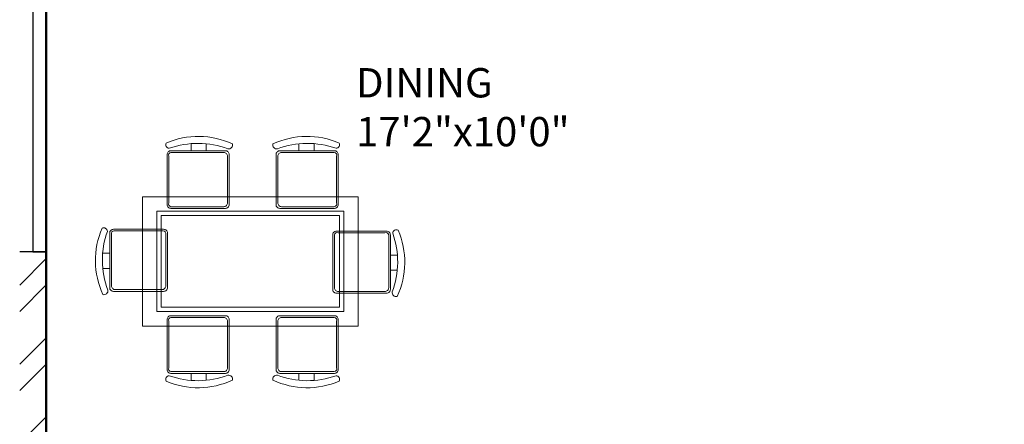
# Model space of a CAD drawing. Units: inches. Extents: x 1901 to 2863, y 888 to 2433.
# Tile 32 of 91: x 2439 to 2607, y 1405 to 1474. Entities that reach past the tile are written whole.
import ezdxf

# ---------------------------------------------------------------- set-up
doc = ezdxf.new("R2010")
doc.units = ezdxf.units.IN
for name, color, linetype, lineweight in [('A-AREA-IDEN', 7, 'Continuous', 18), ('A-FURN', 8, 'Continuous', 18), ('A-GLAZ', 3, 'Continuous', 25), ('A-WALL', 7, 'Continuous', 50), ('A-WALL-PATT', 8, 'Continuous', 13)]:
    doc.layers.add(name, color=color, linetype=linetype, lineweight=lineweight)
doc.styles.get("Standard").update_dxf_attribs({"font": 'arial.ttf'})

# ---------------------------------------------------------------- blocks, each defined once
blk = doc.blocks.new('WIN-60')
for p, q in [((0, 4.5), (0, 0)), ((60, 2.25), (60, 4.5)), ((60, 4.5), (60, 0)), ((0, 0), (0, 2.25)), ((0, 2.25), (60, 2.25))]:
    blk.add_line(p, q)

msp = doc.modelspace()

# ---------------------------------------------------------------- hatches: boundary and pattern name
at = {"layer": 'A-WALL-PATT'}
h = msp.add_hatch(dxfattribs=at)
h.set_pattern_fill('ANSI32', color=256)
h.paths.add_polyline_path([(2192.5, 2274.13), (2141.26, 2274.13), (2141.26, 2269.63), (2192.5, 2269.63)])
h.paths.add_polyline_path([(2259.93, 2274.13), (2216.5, 2274.13), (2216.5, 2269.63), (2255.43, 2269.63), (2255.43, 2214.63), (2250.81, 2214.63), (2250.81, 2210.13), (2259.93, 2210.13), (2259.93, 2215.13), (2271.76, 2215.13), (2271.76, 2217.38), (2271.76, 2219.63), (2259.93, 2219.63)])
h.paths.add_polyline_path([(2171.43, 2269.63), (2166.93, 2269.63), (2166.93, 2219.63), (2121.24, 2219.63), (2121.24, 2215.13), (2166.93, 2215.13), (2166.93, 2083.13), (2161.81, 2083.13), (2161.81, 2078.63), (2171.43, 2078.63), (2177, 2078.63), (2177, 2080.88), (2177, 2083.13), (2171.43, 2083.13), (2171.43, 2210.13), (2230.91, 2210.13), (2230.91, 2212.38), (2230.91, 2214.63), (2171.43, 2214.63)])
h.paths.add_polyline_path([(2117.26, 2274.13), (2089.43, 2274.13), (2089.43, 2219.63), (2081.14, 2219.63), (2081.14, 2215.13), (2089.43, 2215.13), (2098, 2215.13), (2098, 2217.38), (2098, 2219.63), (2093.93, 2219.63), (2093.93, 2269.63), (2117.26, 2269.63), (2117.26, 2271.88)])
h.paths.add_polyline_path([(2343.43, 2219.63), (2329.29, 2219.63), (2329.29, 2215.13), (2338.93, 2215.13), (2338.93, 2184.74), (2343.43, 2184.74)])
h.paths.add_polyline_path([(2338.93, 2083.13), (2329.29, 2083.13), (2208.97, 2083.13), (2208.97, 2078.63), (2338.93, 2078.63)])
h.paths.add_polyline_path([(2343.43, 2136.74), (2338.93, 2136.74), (2338.93, 1872.63), (2343.43, 1872.63)])
h.paths.add_polyline_path([(2343.43, 1863.63), (2397.68, 1863.63), (2397.68, 1821.63), (2384.14, 1821.63), (2384.14, 1812.63), (2418.33, 1812.63), (2418.33, 1817.13), (2418.33, 1821.63), (2406.68, 1821.63), (2406.68, 1863.63), (2459.5, 1863.63), (2459.5, 1821.63), (2447.14, 1821.63), (2447.14, 1812.63), (2459.5, 1812.63), (2468.5, 1812.63), (2468.5, 1872.63), (2394.43, 1872.63), (2334.43, 1872.63), (2334.43, 1812.63), (2343.43, 1812.63), (2353.25, 1812.63), (2353.25, 1821.63), (2343.43, 1821.63)])
h.paths.add_polyline_path([(2510.01, 1872.63), (2468.5, 1872.63), (2468.5, 1868.13), (2510.01, 1868.13)])
h.paths.add_polyline_path([(2514.01, 1817.13), (2468.5, 1817.13), (2468.5, 1812.63), (2482.11, 1812.63), (2482.11, 1800.61), (2486.61, 1800.61), (2486.61, 1812.63), (2514.01, 1812.63)])
h.paths.add_polyline_path([(2299.25, 1814.88), (2299.25, 1817.13), (2295.93, 1817.13), (2295.93, 1854.17), (2293.68, 1854.17), (2291.43, 1854.17), (2291.43, 1817.13), (2266.11, 1817.13), (2266.11, 1812.63), (2299.25, 1812.63)])
h.paths.add_polyline_path([(2218.11, 1817.13), (2206.46, 1817.13), (2171.43, 1817.13), (2171.43, 1949.13), (2190.1, 1949.13), (2190.1, 1953.63), (2163.47, 1953.63), (2163.47, 1949.13), (2166.93, 1949.13), (2166.93, 1817.13), (2114.3, 1817.13), (2114.3, 1812.63), (2218.11, 1812.63)])
h.paths.add_polyline_path([(2029.43, 1970.92), (2024.93, 1970.92), (2024.93, 1912.72), (2029.43, 1912.72)])
h.paths.add_polyline_path([(2132.3, 1953.63), (2113.93, 1953.63), (2113.93, 1975.89), (2111.68, 1975.89), (2109.43, 1975.89), (2109.43, 1953.63), (2029.43, 1953.63), (2029.43, 1949.13), (2132.3, 1949.13)])
h.paths.add_polyline_path([(2029.43, 1853.61), (2029.31, 1853.61), (2029.31, 1853.61), (2029.43, 1853.61), (2029.43, 1864.72), (2024.93, 1864.72), (2024.93, 1812.63), (2066.3, 1812.63), (2066.3, 1814.88), (2066.3, 1817.13), (2029.43, 1817.13)])
h.paths.add_polyline_path([(2122.93, 2010.09), (2120.68, 2010.09), (2118.43, 2010.09), (2118.43, 2006.13), (2029.43, 2006.13), (2029.43, 2001.63), (2109.43, 2001.63), (2109.43, 1998.04), (2113.93, 1998.04), (2113.93, 2001.63), (2122.93, 2001.63)])
h.paths.add_polyline_path([(2029.43, 2031.38), (2024.93, 2031.38), (2024.93, 1994.92), (2027.18, 1994.92), (2029.43, 1994.92)])
h.paths.add_polyline_path([(2029.43, 2136.74), (2024.93, 2136.74), (2024.93, 2067.38), (2027.18, 2067.38), (2029.43, 2067.38)])
h.paths.add_polyline_path([(2125.62, 2083.13), (2029.43, 2083.13), (2029.43, 2078.63), (2118.43, 2078.63), (2118.43, 2030.71), (2122.93, 2030.71), (2122.93, 2078.63), (2125.62, 2078.63)])
h.paths.add_polyline_path([(2029.43, 2215.13), (2040.47, 2215.13), (2040.47, 2217.38), (2040.47, 2219.63), (2024.93, 2219.63), (2024.93, 2184.74), (2029.43, 2184.74), (2029.43, 2187.78)])
h.paths.add_polyline_path([(2686.43, 2274.13), (2659.28, 2274.13), (2659.28, 2269.63), (2681.93, 2269.63), (2681.93, 2219.63), (2676.82, 2219.63), (2676.82, 2215.13), (2681.93, 2215.13), (2697.01, 2215.13), (2697.01, 2217.38), (2697.01, 2219.63), (2686.43, 2219.63)])
h.paths.add_polyline_path([(2609.93, 2269.63), (2635.28, 2269.63), (2635.28, 2274.13), (2571.43, 2274.13), (2571.43, 2269.63), (2605.43, 2269.63), (2605.43, 2214.63), (2549.1, 2214.63), (2549.1, 2210.13), (2605.43, 2210.13), (2605.43, 2083.13), (2601.01, 2083.13), (2601.01, 2080.88), (2601.01, 2078.63), (2609.93, 2078.63), (2616.16, 2078.63), (2616.16, 2080.88), (2616.16, 2083.13), (2609.93, 2083.13), (2609.93, 2215.13), (2651.46, 2215.13), (2651.46, 2217.38), (2651.46, 2219.63), (2609.93, 2219.63)])
h.paths.add_polyline_path([(2521.43, 2269.63), (2547.43, 2269.63), (2547.43, 2271.88), (2547.43, 2274.13), (2516.93, 2274.13), (2516.93, 2219.63), (2506.41, 2219.63), (2506.41, 2215.13), (2516.93, 2215.13), (2516.93, 2210.13), (2525.4, 2210.13), (2525.4, 2212.38), (2525.4, 2214.63), (2521.43, 2214.63)])
h.paths.add_polyline_path([(2456.01, 2219.63), (2439.43, 2219.63), (2439.43, 2187.89), (2443.93, 2187.89), (2443.93, 2215.13), (2456.01, 2215.13)])
h.paths.add_polyline_path([(2752.93, 2219.63), (2739.48, 2219.63), (2739.48, 2215.13), (2748.43, 2215.13), (2748.43, 2187.89), (2752.93, 2187.89)])
h.paths.add_polyline_path([(2752.93, 2139.89), (2748.43, 2139.89), (2748.43, 2083.13), (2648.42, 2083.13), (2648.42, 2078.63), (2654.93, 2078.63), (2654.93, 2039.44), (2659.43, 2039.44), (2659.43, 2078.63), (2748.43, 2078.63), (2748.43, 2063.43), (2752.93, 2063.43)])
h.paths.add_polyline_path([(2752.93, 2010.63), (2659.43, 2010.63), (2659.43, 2015.65), (2654.93, 2015.65), (2654.93, 2010.63), (2605.43, 2010.63), (2605.43, 1920.97), (2609.93, 1920.97), (2609.93, 2006.13), (2748.43, 2006.13), (2748.43, 1982.47), (2752.93, 1982.47)])
h.paths.add_polyline_path([(2752.93, 2027.43), (2748.43, 2027.43), (2748.43, 2010.63), (2752.93, 2010.63)])
h.paths.add_polyline_path([(2748.43, 1886.13), (2609.93, 1886.13), (2609.93, 1889.72), (2605.43, 1889.72), (2605.43, 1861.26), (2609.93, 1861.26), (2609.93, 1881.63), (2748.43, 1881.63)])
h.paths.add_polyline_path([(2456.86, 2228.83), (2498.4, 2228.83), (2498.4, 2247.49), (2456.86, 2247.49)], flags=9)
h.paths.add_polyline_path([(2038.6, 2237.42), (2080.17, 2237.42), (2080.17, 2256.08), (2038.6, 2256.08)], flags=9)
h.paths.add_polyline_path([(2292.01, 1062.39), (2539.93, 1062.39), (2539.93, 1099.49), (2292.01, 1099.49)], flags=9)
h.paths.add_polyline_path([(2424.91, 1832.25), (2448.51, 1832.25), (2448.51, 1846.68), (2424.91, 1846.68)], flags=25)
h.paths.add_polyline_path([(2359.08, 1832.25), (2382.68, 1832.25), (2382.68, 1846.68), (2359.08, 1846.68)], flags=25)
h.paths.add_polyline_path([(2352.9, 1684.8), (2367.54, 1684.8), (2367.54, 1697.17), (2352.9, 1697.17)], flags=9)
h.paths.add_polyline_path([(2079.29, 1755.83), (2169.02, 1755.83), (2169.02, 1774.37), (2079.29, 1774.37)], flags=9)
h.paths.add_polyline_path([(2404.09, 1373.86), (2404.09, 1463.59), (2385.54, 1463.59), (2385.54, 1373.86)], flags=9)
h.paths.add_polyline_path([(2268.09, 2236.37), (2309.64, 2236.37), (2309.64, 2255.03), (2268.09, 2255.03)], flags=9)
h.paths.add_polyline_path([(2575.96, 1700.95), (2665.7, 1700.95), (2665.7, 1719.5), (2575.96, 1719.5)], flags=9)
h.paths.add_polyline_path([(2302.96, 1878.47), (2329.52, 1878.47), (2329.52, 1888.78), (2302.96, 1888.78)], flags=9)
h.paths.add_polyline_path([(2097.42, 2240.58), (2126.57, 2240.58), (2126.57, 2259.23), (2097.42, 2259.23)], flags=9)
h.paths.add_polyline_path([(2208.72, 2246.12), (2237.88, 2246.12), (2237.88, 2264.78), (2208.72, 2264.78)], flags=9)
h.paths.add_polyline_path([(2038.15, 1925.96), (2076.99, 1925.96), (2076.99, 1944.62), (2038.15, 1944.62)], flags=9)
h.paths.add_polyline_path([(2239.14, 1926.67), (2288.46, 1926.67), (2288.46, 1945.33), (2239.14, 1945.33)], flags=9)
h.paths.add_polyline_path([(2175.43, 2007.33), (2212.36, 2007.33), (2212.36, 2025.99), (2175.43, 2025.99)], flags=9)
h.paths.add_polyline_path([(2225.03, 2091.79), (2263.87, 2091.79), (2263.87, 2110.45), (2225.03, 2110.45)], flags=9)
h.paths.add_polyline_path([(2035.4, 2098.48), (2074.24, 2098.48), (2074.24, 2117.14), (2035.4, 2117.14)], flags=9)
h.paths.add_polyline_path([(2050.1, 2029.21), (2083.26, 2029.21), (2083.26, 2047.87), (2050.1, 2047.87)], flags=9)
h.paths.add_polyline_path([(2069.68, 1956.72), (2098.83, 1956.72), (2098.83, 1975.38), (2069.68, 1975.38)], flags=25)
h.paths.add_polyline_path([(2328.62, 1753.34), (2361.66, 1753.34), (2361.66, 1771.99), (2328.62, 1771.99)], flags=9)
h.paths.add_polyline_path([(2395.16, 2060.89), (2395.16, 2140.65), (2378.68, 2140.65), (2378.68, 2060.89)], flags=9)
h.paths.add_polyline_path([(2463.73, 2059.02), (2492.89, 2059.02), (2492.89, 2077.68), (2463.73, 2077.68)], flags=9)
h.paths.add_polyline_path([(2458.03, 2181.54), (2496.87, 2181.54), (2496.87, 2200.19), (2458.03, 2200.19)], flags=9)
h.paths.add_polyline_path([(2527.58, 2243.07), (2556.73, 2243.07), (2556.73, 2261.73), (2527.58, 2261.73)], flags=9)
h.paths.add_polyline_path([(2694.46, 2232.77), (2736.03, 2232.77), (2736.03, 2251.42), (2694.46, 2251.42)], flags=9)
h.paths.add_polyline_path([(2637.82, 2249.22), (2666.98, 2249.22), (2666.98, 2267.88), (2637.82, 2267.88)], flags=9)
h.paths.add_polyline_path([(2623.69, 2183.54), (2662.53, 2183.54), (2662.53, 2202.2), (2623.69, 2202.2)], flags=9)
h.paths.add_polyline_path([(2691.97, 2021.5), (2725.12, 2021.5), (2725.12, 2040.16), (2691.97, 2040.16)], flags=9)
h.paths.add_polyline_path([(2621.04, 1975.91), (2662.34, 1975.91), (2662.34, 1994.57), (2621.04, 1994.57)], flags=25)
h.paths.add_polyline_path([(2479.03, 1927.62), (2519.84, 1927.62), (2519.84, 1946.28), (2479.03, 1946.28)], flags=9)
h.paths.add_polyline_path([(2670.94, 1849.08), (2716.01, 1849.08), (2716.01, 1867.73), (2670.94, 1867.73)], flags=9)
h.paths.add_polyline_path([(2523.61, 1782.96), (2550.17, 1782.96), (2550.17, 1793.26), (2523.61, 1793.26)], flags=9)
h.paths.add_polyline_path([(2450.84, 1207.33), (2492.39, 1207.33), (2492.39, 1225.99), (2450.84, 1225.99)], flags=9)
h.paths.add_polyline_path([(2527.75, 1203.84), (2556.91, 1203.84), (2556.91, 1222.5), (2527.75, 1222.5)], flags=9)
h.paths.add_polyline_path([(2639.11, 1207.2), (2668.27, 1207.2), (2668.27, 1225.86), (2639.11, 1225.86)], flags=9)
h.paths.add_polyline_path([(2692.59, 1218.97), (2734.17, 1218.97), (2734.17, 1237.62), (2692.59, 1237.62)], flags=9)
h.paths.add_polyline_path([(2669.27, 1366.33), (2708.11, 1366.33), (2708.11, 1384.99), (2669.27, 1384.99)], flags=9)
h.paths.add_polyline_path([(2463.31, 1358.03), (2502.15, 1358.03), (2502.15, 1376.69), (2463.31, 1376.69)], flags=9)
h.paths.add_polyline_path([(2494.72, 1449.96), (2531.65, 1449.96), (2531.65, 1468.62), (2494.72, 1468.62)], flags=9)
h.paths.add_polyline_path([(2675.57, 1422.16), (2708.72, 1422.16), (2708.72, 1440.81), (2675.57, 1440.81)], flags=9)
h.paths.add_polyline_path([(2685.63, 1493.89), (2714.79, 1493.89), (2714.79, 1512.55), (2685.63, 1512.55)], flags=9)
h.paths.add_polyline_path([(2686.8, 1529.91), (2725.65, 1529.91), (2725.65, 1548.57), (2686.8, 1548.57)], flags=9)
h.paths.add_polyline_path([(2503.65, 1537.99), (2552.97, 1537.99), (2552.97, 1556.65), (2503.65, 1556.65)], flags=9)
h.paths.add_polyline_path([(2291.71, 1643.5), (2318.28, 1643.5), (2318.28, 1653.81), (2291.71, 1653.81)], flags=9)
h.paths.add_polyline_path([(2450.63, 1610.52), (2477.19, 1610.52), (2477.19, 1620.82), (2450.63, 1620.82)], flags=9)
h.paths.add_polyline_path([(2359.99, 1551.81), (2422.25, 1551.81), (2422.25, 1562.12), (2359.99, 1562.12)], flags=9)
h.paths.add_polyline_path([(2280.11, 1249.01), (2321.65, 1249.01), (2321.65, 1267.66), (2280.11, 1267.66)], flags=9)
h.paths.add_polyline_path([(2164.06, 1274.23), (2193.22, 1274.23), (2193.22, 1292.89), (2164.06, 1292.89)], flags=9)
h.paths.add_polyline_path([(2118.21, 1277.69), (2151.25, 1277.69), (2151.25, 1296.35), (2118.21, 1296.35)], flags=9)
h.paths.add_polyline_path([(2031.95, 1268.53), (2073.52, 1268.53), (2073.52, 1287.19), (2031.95, 1287.19)], flags=9)
h.paths.add_polyline_path([(2050.2, 1409.08), (2089.04, 1409.08), (2089.04, 1427.74), (2050.2, 1427.74)], flags=9)
h.paths.add_polyline_path([(2243.74, 1421.03), (2282.58, 1421.03), (2282.58, 1439.69), (2243.74, 1439.69)], flags=9)
h.paths.add_polyline_path([(2190.75, 1509.77), (2231.56, 1509.77), (2231.56, 1528.43), (2190.75, 1528.43)], flags=9)
h.paths.add_polyline_path([(2058.39, 1475.42), (2091.55, 1475.42), (2091.55, 1494.07), (2058.39, 1494.07)], flags=9)
h.paths.add_polyline_path([(2062.45, 1553.09), (2091.6, 1553.09), (2091.6, 1571.75), (2062.45, 1571.75)], flags=9)
h.paths.add_polyline_path([(2219.52, 1590.37), (2266.15, 1590.37), (2266.15, 1609.02), (2219.52, 1609.02)], flags=9)
h.paths.add_polyline_path([(2041.07, 1584.19), (2079.91, 1584.19), (2079.91, 1602.85), (2041.07, 1602.85)], flags=9)
h = msp.add_hatch(dxfattribs=at)
h.set_pattern_fill('ANSI32', color=256)
h.paths.add_polyline_path([(2443.93, 2139.89), (2439.43, 2139.89), (2439.43, 2069.35), (2441.68, 2069.35), (2443.93, 2069.35), (2443.93, 2078.63), (2521.93, 2078.63), (2521.93, 2075.07), (2524.18, 2075.07), (2526.43, 2075.07), (2526.43, 2078.63), (2571.75, 2078.63), (2571.75, 2080.88), (2571.75, 2083.13), (2443.93, 2083.13)])
h.paths.add_polyline_path([(2526.43, 2054.63), (2524.18, 2054.63), (2521.93, 2054.63), (2521.93, 2030.63), (2443.93, 2030.63), (2443.93, 2045.35), (2439.43, 2045.35), (2439.43, 1983.87), (2443.93, 1983.87), (2443.93, 2026.13), (2521.93, 2026.13), (2526.43, 2026.13)])
h.paths.add_polyline_path([(2443.93, 1923.87), (2439.43, 1923.87), (2439.43, 1872.63), (2443.93, 1872.63)])
h.paths.add_polyline_path([(2636.23, 1766.13), (2609.93, 1766.13), (2609.93, 1779.79), (2605.43, 1779.79), (2605.43, 1766.13), (2486.61, 1766.13), (2486.61, 1770.67), (2482.11, 1770.67), (2482.11, 1766.13), (2482.11, 1761.63), (2636.23, 1761.63), (2636.23, 1763.88)])
h.paths.add_polyline_path([(2519.54, 1663.38), (2519.54, 1665.63), (2494.93, 1665.63), (2481.83, 1665.63), (2481.83, 1663.38), (2481.83, 1661.13), (2490.43, 1661.13), (2490.43, 1640.16), (2494.93, 1640.16), (2494.93, 1661.13), (2519.54, 1661.13)])
h.paths.add_polyline_path([(2443.93, 1712.13), (2443.93, 1716.63), (2414.46, 1716.63), (2414.46, 1712.13), (2439.43, 1712.13), (2439.43, 1545.51), (2443.93, 1545.51), (2443.93, 1661.13), (2448.47, 1661.13), (2448.47, 1665.63), (2443.93, 1665.63)])
h.paths.add_polyline_path([(2343.43, 1712.13), (2365.52, 1712.13), (2365.52, 1714.38), (2365.52, 1716.63), (2333.87, 1716.63), (2333.87, 1714.38), (2333.87, 1712.13), (2338.93, 1712.13), (2338.93, 1575.63), (2338.93, 1545.51), (2343.43, 1545.51), (2343.43, 1547.51), (2343.43, 1580.13)])
h.paths.add_polyline_path([(2752.93, 1665.63), (2579.54, 1665.63), (2579.54, 1661.13), (2615.93, 1661.13), (2615.93, 1529.13), (2598.93, 1529.13), (2598.93, 1524.63), (2623.13, 1524.63), (2623.13, 1526.88), (2623.13, 1529.13), (2620.43, 1529.13), (2620.43, 1661.13), (2748.43, 1661.13), (2748.43, 1633.5), (2752.93, 1633.5)])
h.paths.add_polyline_path([(2752.93, 1419.93), (2748.43, 1419.93), (2748.43, 1400.13), (2659.43, 1400.13), (2659.43, 1444.33), (2657.18, 1444.33), (2654.93, 1444.33), (2654.93, 1400.13), (2643.65, 1400.13), (2643.65, 1395.63), (2748.43, 1395.63), (2748.43, 1364.04), (2752.93, 1364.04)])
h.paths.add_polyline_path([(2752.93, 1492.88), (2748.43, 1492.88), (2748.43, 1476.63), (2667.43, 1476.63), (2667.43, 1479.71), (2665.18, 1479.71), (2662.93, 1479.71), (2662.93, 1476.63), (2654.93, 1476.63), (2654.93, 1469.54), (2659.43, 1469.54), (2659.43, 1472.13), (2748.43, 1472.13), (2748.43, 1455.93), (2752.93, 1455.93)])
h.paths.add_polyline_path([(2752.93, 1304.04), (2748.43, 1304.04), (2748.43, 1263.63), (2738.66, 1263.63), (2738.66, 1259.13), (2752.93, 1259.13)])
h.paths.add_polyline_path([(2685.93, 1259.13), (2695.49, 1259.13), (2695.49, 1261.38), (2695.49, 1263.63), (2677.84, 1263.63), (2677.84, 1261.38), (2677.84, 1259.13), (2681.43, 1259.13), (2681.43, 1203.63), (2653.28, 1203.63), (2653.28, 1199.13), (2685.93, 1199.13), (2685.93, 1203.63)])
h.paths.add_polyline_path([(2609.43, 1395.63), (2611.85, 1395.63), (2611.85, 1400.13), (2598.89, 1400.13), (2598.89, 1397.88), (2598.89, 1395.63), (2604.93, 1395.63), (2604.93, 1268.13), (2554.73, 1268.13), (2554.73, 1265.88), (2554.73, 1263.63), (2604.93, 1263.63), (2604.93, 1203.63), (2571.31, 1203.63), (2571.31, 1199.13), (2604.93, 1199.13), (2629.28, 1199.13), (2629.28, 1201.38), (2629.28, 1203.63), (2609.43, 1203.63), (2609.43, 1258.63), (2609.43, 1259.13), (2654.8, 1259.13), (2654.8, 1263.63), (2609.43, 1263.63)])
h.paths.add_polyline_path([(2443.93, 1304.04), (2439.43, 1304.04), (2439.43, 1259.13), (2443.93, 1259.13), (2456.16, 1259.13), (2456.16, 1261.38), (2456.16, 1263.63), (2443.93, 1263.63)])
h.paths.add_polyline_path([(2525.43, 1263.63), (2531.78, 1263.63), (2531.78, 1268.13), (2520.93, 1268.13), (2520.93, 1263.63), (2511.41, 1263.63), (2511.41, 1259.13), (2520.93, 1259.13), (2520.93, 1199.13), (2547.31, 1199.13), (2547.31, 1201.38), (2547.31, 1203.63), (2525.43, 1203.63)])
h.paths.add_polyline_path([(2443.93, 1434.84), (2439.43, 1434.84), (2439.43, 1364.04), (2441.68, 1364.04), (2443.93, 1364.04)])
h.paths.add_polyline_path([(2567.13, 1400.13), (2443.93, 1400.13), (2443.93, 1395.63), (2567.13, 1395.63)])
h.paths.add_polyline_path([(2443.93, 1545.51), (2439.43, 1545.51), (2439.43, 1494.84), (2443.93, 1494.84)])
h.paths.add_polyline_path([(2494.93, 1553.35), (2492.68, 1553.35), (2490.43, 1553.35), (2490.43, 1524.63), (2494.93, 1524.63), (2525.94, 1524.63), (2525.94, 1526.88), (2525.94, 1529.13), (2494.93, 1529.13)])
h.paths.add_polyline_path([(2752.93, 1573.5), (2748.43, 1573.5), (2748.43, 1529.13), (2657.76, 1529.13), (2657.76, 1524.63), (2662.93, 1524.63), (2662.93, 1498.63), (2667.43, 1498.63), (2667.43, 1524.63), (2748.43, 1524.63), (2748.43, 1516.88), (2752.93, 1516.88)])
h.paths.add_polyline_path([(2038.6, 2237.42), (2080.17, 2237.42), (2080.17, 2256.08), (2038.6, 2256.08)], flags=9)
h.paths.add_polyline_path([(2292.01, 1062.39), (2539.93, 1062.39), (2539.93, 1099.49), (2292.01, 1099.49)], flags=9)
h.paths.add_polyline_path([(2424.91, 1832.25), (2448.51, 1832.25), (2448.51, 1846.68), (2424.91, 1846.68)], flags=9)
h.paths.add_polyline_path([(2359.08, 1832.25), (2382.68, 1832.25), (2382.68, 1846.68), (2359.08, 1846.68)], flags=9)
h.paths.add_polyline_path([(2352.9, 1684.8), (2367.54, 1684.8), (2367.54, 1697.17), (2352.9, 1697.17)], flags=9)
h.paths.add_polyline_path([(2079.29, 1755.83), (2169.02, 1755.83), (2169.02, 1774.37), (2079.29, 1774.37)], flags=9)
h.paths.add_polyline_path([(2404.09, 1373.86), (2404.09, 1463.59), (2385.54, 1463.59), (2385.54, 1373.86)], flags=9)
h.paths.add_polyline_path([(2268.09, 2236.37), (2309.64, 2236.37), (2309.64, 2255.03), (2268.09, 2255.03)], flags=9)
h.paths.add_polyline_path([(2575.96, 1700.95), (2665.7, 1700.95), (2665.7, 1719.5), (2575.96, 1719.5)], flags=9)
h.paths.add_polyline_path([(2302.96, 1878.47), (2329.52, 1878.47), (2329.52, 1888.78), (2302.96, 1888.78)], flags=9)
h.paths.add_polyline_path([(2097.42, 2240.58), (2126.57, 2240.58), (2126.57, 2259.23), (2097.42, 2259.23)], flags=9)
h.paths.add_polyline_path([(2208.72, 2246.12), (2237.88, 2246.12), (2237.88, 2264.78), (2208.72, 2264.78)], flags=9)
h.paths.add_polyline_path([(2038.15, 1925.96), (2076.99, 1925.96), (2076.99, 1944.62), (2038.15, 1944.62)], flags=9)
h.paths.add_polyline_path([(2239.14, 1926.67), (2288.46, 1926.67), (2288.46, 1945.33), (2239.14, 1945.33)], flags=9)
h.paths.add_polyline_path([(2175.43, 2007.33), (2212.36, 2007.33), (2212.36, 2025.99), (2175.43, 2025.99)], flags=9)
h.paths.add_polyline_path([(2225.03, 2091.79), (2263.87, 2091.79), (2263.87, 2110.45), (2225.03, 2110.45)], flags=9)
h.paths.add_polyline_path([(2035.4, 2098.48), (2074.24, 2098.48), (2074.24, 2117.14), (2035.4, 2117.14)], flags=9)
h.paths.add_polyline_path([(2050.1, 2029.21), (2083.26, 2029.21), (2083.26, 2047.87), (2050.1, 2047.87)], flags=9)
h.paths.add_polyline_path([(2069.68, 1956.72), (2098.83, 1956.72), (2098.83, 1975.38), (2069.68, 1975.38)], flags=9)
h.paths.add_polyline_path([(2328.62, 1753.34), (2361.66, 1753.34), (2361.66, 1771.99), (2328.62, 1771.99)], flags=9)
h.paths.add_polyline_path([(2395.16, 2060.89), (2395.16, 2140.65), (2378.68, 2140.65), (2378.68, 2060.89)], flags=9)
h.paths.add_polyline_path([(2463.73, 2059.02), (2492.89, 2059.02), (2492.89, 2077.68), (2463.73, 2077.68)], flags=9)
h.paths.add_polyline_path([(2458.03, 2181.54), (2496.87, 2181.54), (2496.87, 2200.19), (2458.03, 2200.19)], flags=9)
h.paths.add_polyline_path([(2456.86, 2228.83), (2498.4, 2228.83), (2498.4, 2247.49), (2456.86, 2247.49)], flags=9)
h.paths.add_polyline_path([(2527.58, 2243.07), (2556.73, 2243.07), (2556.73, 2261.73), (2527.58, 2261.73)], flags=9)
h.paths.add_polyline_path([(2694.46, 2232.77), (2736.03, 2232.77), (2736.03, 2251.42), (2694.46, 2251.42)], flags=9)
h.paths.add_polyline_path([(2637.82, 2249.22), (2666.98, 2249.22), (2666.98, 2267.88), (2637.82, 2267.88)], flags=9)
h.paths.add_polyline_path([(2623.69, 2183.54), (2662.53, 2183.54), (2662.53, 2202.2), (2623.69, 2202.2)], flags=9)
h.paths.add_polyline_path([(2691.97, 2021.5), (2725.12, 2021.5), (2725.12, 2040.16), (2691.97, 2040.16)], flags=9)
h.paths.add_polyline_path([(2621.04, 1975.91), (2662.34, 1975.91), (2662.34, 1994.57), (2621.04, 1994.57)], flags=9)
h.paths.add_polyline_path([(2479.03, 1927.62), (2519.84, 1927.62), (2519.84, 1946.28), (2479.03, 1946.28)], flags=9)
h.paths.add_polyline_path([(2670.94, 1849.08), (2716.01, 1849.08), (2716.01, 1867.73), (2670.94, 1867.73)], flags=9)
h.paths.add_polyline_path([(2523.61, 1782.96), (2550.17, 1782.96), (2550.17, 1793.26), (2523.61, 1793.26)], flags=9)
h.paths.add_polyline_path([(2450.84, 1207.33), (2492.39, 1207.33), (2492.39, 1225.99), (2450.84, 1225.99)], flags=9)
h.paths.add_polyline_path([(2527.75, 1203.84), (2556.91, 1203.84), (2556.91, 1222.5), (2527.75, 1222.5)], flags=9)
h.paths.add_polyline_path([(2639.11, 1207.2), (2668.27, 1207.2), (2668.27, 1225.86), (2639.11, 1225.86)], flags=9)
h.paths.add_polyline_path([(2692.59, 1218.97), (2734.17, 1218.97), (2734.17, 1237.62), (2692.59, 1237.62)], flags=9)
h.paths.add_polyline_path([(2669.27, 1366.33), (2708.11, 1366.33), (2708.11, 1384.99), (2669.27, 1384.99)], flags=25)
h.paths.add_polyline_path([(2463.31, 1358.03), (2502.15, 1358.03), (2502.15, 1376.69), (2463.31, 1376.69)], flags=9)
h.paths.add_polyline_path([(2494.72, 1449.96), (2531.65, 1449.96), (2531.65, 1468.62), (2494.72, 1468.62)], flags=9)
h.paths.add_polyline_path([(2675.57, 1422.16), (2708.72, 1422.16), (2708.72, 1440.81), (2675.57, 1440.81)], flags=25)
h.paths.add_polyline_path([(2685.63, 1493.89), (2714.79, 1493.89), (2714.79, 1512.55), (2685.63, 1512.55)], flags=9)
h.paths.add_polyline_path([(2686.8, 1529.91), (2725.65, 1529.91), (2725.65, 1548.57), (2686.8, 1548.57)], flags=25)
h.paths.add_polyline_path([(2503.65, 1537.99), (2552.97, 1537.99), (2552.97, 1556.65), (2503.65, 1556.65)], flags=9)
h.paths.add_polyline_path([(2291.71, 1643.5), (2318.28, 1643.5), (2318.28, 1653.81), (2291.71, 1653.81)], flags=9)
h.paths.add_polyline_path([(2450.63, 1610.52), (2477.19, 1610.52), (2477.19, 1620.82), (2450.63, 1620.82)], flags=9)
h.paths.add_polyline_path([(2359.99, 1551.81), (2422.25, 1551.81), (2422.25, 1562.12), (2359.99, 1562.12)], flags=9)
h.paths.add_polyline_path([(2280.11, 1249.01), (2321.65, 1249.01), (2321.65, 1267.66), (2280.11, 1267.66)], flags=9)
h.paths.add_polyline_path([(2164.06, 1274.23), (2193.22, 1274.23), (2193.22, 1292.89), (2164.06, 1292.89)], flags=9)
h.paths.add_polyline_path([(2118.21, 1277.69), (2151.25, 1277.69), (2151.25, 1296.35), (2118.21, 1296.35)], flags=9)
h.paths.add_polyline_path([(2031.95, 1268.53), (2073.52, 1268.53), (2073.52, 1287.19), (2031.95, 1287.19)], flags=9)
h.paths.add_polyline_path([(2050.2, 1409.08), (2089.04, 1409.08), (2089.04, 1427.74), (2050.2, 1427.74)], flags=9)
h.paths.add_polyline_path([(2243.74, 1421.03), (2282.58, 1421.03), (2282.58, 1439.69), (2243.74, 1439.69)], flags=9)
h.paths.add_polyline_path([(2190.75, 1509.77), (2231.56, 1509.77), (2231.56, 1528.43), (2190.75, 1528.43)], flags=9)
h.paths.add_polyline_path([(2058.39, 1475.42), (2091.55, 1475.42), (2091.55, 1494.07), (2058.39, 1494.07)], flags=9)
h.paths.add_polyline_path([(2062.45, 1553.09), (2091.6, 1553.09), (2091.6, 1571.75), (2062.45, 1571.75)], flags=9)
h.paths.add_polyline_path([(2219.52, 1590.37), (2266.15, 1590.37), (2266.15, 1609.02), (2219.52, 1609.02)], flags=9)
h.paths.add_polyline_path([(2041.07, 1584.19), (2079.91, 1584.19), (2079.91, 1602.85), (2041.07, 1602.85)], flags=9)

# ---------------------------------------------------------------- linework, layer by layer
at = {"layer": 'A-FURN'}
for points in [[(2464.9, 1452.46, -0.175809), (2474.9, 1452.38, 0.578392), (2475.66, 1453.21, 0.214524), (2464.37, 1453.36, 0.552014), (2464.9, 1452.46, -0.065079)], [(2464.9, 1452.46, -0.175809), (2474.9, 1452.38, 0.578392), (2475.66, 1453.21, 0.214524), (2464.37, 1453.36, 0.552014), (2464.9, 1452.46, -0.065079)], [(2483.33, 1452.38, -0.578392), (2482.57, 1453.21, -0.214524), (2493.86, 1453.36, -0.552014), (2493.33, 1452.46, 0.175809), (2483.33, 1452.38)], [(2483.33, 1452.38, -0.578392), (2482.57, 1453.21, -0.214524), (2493.86, 1453.36, -0.552014), (2493.33, 1452.46, 0.175809), (2483.33, 1452.38)], [(2471.22, 1452.05), (2471.22, 1453.23, -0.064759)], [(2471.22, 1452.05), (2471.22, 1453.23, -0.064759)], [(2487.01, 1452.05), (2487.01, 1453.23, 0.064759)], [(2487.01, 1452.05), (2487.01, 1453.23, 0.064759)], [(2474.48, 1452.05), (2465.19, 1452.05, 0.414214), (2464.54, 1451.4), (2464.54, 1442.87, 0.414214), (2465.19, 1442.22), (2474.48, 1442.22, 0.414214), (2475.13, 1442.87), (2475.13, 1451.4, 0.414214), (2474.48, 1452.05)], [(2474.48, 1452.05), (2465.19, 1452.05, 0.414214), (2464.54, 1451.4), (2464.54, 1442.87, 0.414214), (2465.19, 1442.22), (2474.48, 1442.22, 0.414214), (2475.13, 1442.87), (2475.13, 1451.4, 0.414214), (2474.48, 1452.05)], [(2493.04, 1452.05, -0.414214), (2493.69, 1451.4), (2493.69, 1442.87, -0.414214), (2493.04, 1442.22), (2483.75, 1442.22, -0.414214), (2483.1, 1442.87), (2483.1, 1451.4, -0.414214), (2483.75, 1452.05), (2493.04, 1452.05)], [(2493.04, 1452.05, -0.414214), (2493.69, 1451.4), (2493.69, 1442.87, -0.414214), (2493.04, 1442.22), (2483.75, 1442.22, -0.414214), (2483.1, 1442.87), (2483.1, 1451.4, -0.414214), (2483.75, 1452.05), (2493.04, 1452.05)], [(2454.43, 1428.3, -0.578392), (2453.6, 1427.54, -0.214524), (2453.45, 1438.83, -0.552014), (2454.36, 1438.3, 0.175809), (2454.43, 1428.3)], [(2454.43, 1428.3, -0.578392), (2453.6, 1427.54, -0.214524), (2453.45, 1438.83, -0.552014), (2454.36, 1438.3, 0.175809), (2454.43, 1428.3)], [(2454.76, 1438.01, -0.414214), (2455.41, 1438.66), (2463.95, 1438.66, -0.414214), (2464.6, 1438.01), (2464.6, 1428.72, -0.414214), (2463.95, 1428.07), (2455.41, 1428.07, -0.414214), (2454.76, 1428.72), (2454.76, 1438.01)], [(2454.76, 1438.01, -0.414214), (2455.41, 1438.66), (2463.95, 1438.66, -0.414214), (2464.6, 1438.01), (2464.6, 1428.72, -0.414214), (2463.95, 1428.07), (2455.41, 1428.07, -0.414214), (2454.76, 1428.72), (2454.76, 1438.01)], [(2502.58, 1437.69, 0.414214), (2501.93, 1438.34), (2493.39, 1438.34, 0.414214), (2492.75, 1437.69), (2492.75, 1428.41, 0.414214), (2493.39, 1427.76), (2501.93, 1427.76, 0.414214), (2502.58, 1428.41), (2502.58, 1437.69)], [(2502.58, 1437.69, 0.414214), (2501.93, 1438.34), (2493.39, 1438.34, 0.414214), (2492.75, 1437.69), (2492.75, 1428.4, 0.414214), (2493.39, 1427.75), (2501.93, 1427.75, 0.414214), (2502.58, 1428.4), (2502.58, 1437.69)], [(2502.99, 1437.98, -0.175809), (2502.91, 1427.98, 0.578392), (2503.74, 1427.22, 0.214524), (2503.89, 1438.51, 0.552014), (2502.99, 1437.98, -0.065079)], [(2502.99, 1437.98, -0.175809), (2502.91, 1427.98, 0.578392), (2503.74, 1427.22, 0.214524), (2503.89, 1438.51, 0.552014), (2502.99, 1437.98, -0.065079)], [(2454.76, 1431.99), (2453.59, 1431.99, 0.064759)], [(2454.76, 1431.98), (2453.59, 1431.98, 0.064759)], [(2502.58, 1431.67), (2503.76, 1431.67, -0.064759)], [(2502.58, 1431.67), (2503.76, 1431.67, -0.064759)], [(2474.48, 1414.1), (2465.19, 1414.1, -0.414214), (2464.54, 1414.75), (2464.54, 1423.28, -0.414214), (2465.19, 1423.93), (2474.48, 1423.93, -0.414214), (2475.13, 1423.28), (2475.13, 1414.75, -0.414214), (2474.48, 1414.1)], [(2474.48, 1414.1), (2465.19, 1414.1, -0.414214), (2464.54, 1414.74), (2464.54, 1423.28, -0.414214), (2465.19, 1423.93), (2474.48, 1423.93, -0.414214), (2475.13, 1423.28), (2475.13, 1414.74, -0.414214), (2474.48, 1414.1)], [(2493.04, 1414.1, 0.414214), (2493.69, 1414.75), (2493.69, 1423.28, 0.414214), (2493.04, 1423.93), (2483.75, 1423.93, 0.414214), (2483.1, 1423.28), (2483.1, 1414.75, 0.414214), (2483.75, 1414.1), (2493.04, 1414.1)], [(2493.04, 1414.1, 0.414214), (2493.69, 1414.74), (2493.69, 1423.28, 0.414214), (2493.04, 1423.93), (2483.75, 1423.93, 0.414214), (2483.1, 1423.28), (2483.1, 1414.74, 0.414214), (2483.75, 1414.1), (2493.04, 1414.1)], [(2474.9, 1413.77, -0.578392), (2475.66, 1412.94, -0.214524), (2464.37, 1412.78, -0.552014), (2464.9, 1413.69, 0.175809), (2474.9, 1413.77)], [(2474.9, 1413.77, -0.578392), (2475.66, 1412.94, -0.214524), (2464.37, 1412.78, -0.552014), (2464.9, 1413.69, 0.175809), (2474.9, 1413.77)], [(2471.22, 1414.1), (2471.22, 1412.92, 0.064759)], [(2471.22, 1414.1), (2471.22, 1412.92, 0.064759)], [(2493.33, 1413.69, -0.175809), (2483.33, 1413.77, 0.578392), (2482.57, 1412.94, 0.214524), (2493.86, 1412.78, 0.552014), (2493.33, 1413.69, -0.065079)], [(2493.33, 1413.69, -0.175809), (2483.33, 1413.77, 0.578392), (2482.57, 1412.94, 0.214524), (2493.86, 1412.78, 0.552014), (2493.33, 1413.69, -0.065079)], [(2487.01, 1414.1), (2487.01, 1412.92, -0.064759)], [(2487.01, 1414.1), (2487.01, 1412.92, -0.064759)]]:
    msp.add_lwpolyline(points, format="xyb", dxfattribs=at)
for points in [[(2468.62, 1453.25), (2468.62, 1452.05)], [(2468.62, 1453.25), (2468.62, 1452.05)], [(2489.61, 1453.25), (2489.61, 1452.05)], [(2489.61, 1453.25), (2489.61, 1452.05)], [(2453.56, 1434.58), (2454.76, 1434.58)], [(2453.56, 1434.58), (2454.76, 1434.58)], [(2503.78, 1434.27), (2502.58, 1434.27)], [(2503.78, 1434.27), (2502.58, 1434.27)], [(2468.62, 1412.9), (2468.62, 1414.1)], [(2468.62, 1412.9), (2468.62, 1414.1)], [(2489.61, 1412.9), (2489.61, 1414.1)], [(2489.61, 1412.9), (2489.61, 1414.1)]]:
    msp.add_lwpolyline(points, dxfattribs=at)
for points in [[(2465.2, 1451.76), (2474.19, 1451.76, -0.414214), (2474.84, 1451.11), (2474.84, 1443.16, -0.414214), (2474.19, 1442.51), (2465.2, 1442.51, -0.512069), (2464.84, 1443.16), (2464.84, 1451.11, -0.512069)], [(2465.2, 1451.76), (2474.19, 1451.76, -0.414214), (2474.84, 1451.11), (2474.84, 1443.16, -0.414214), (2474.19, 1442.51), (2465.2, 1442.51, -0.512069), (2464.84, 1443.16), (2464.84, 1451.11, -0.512069)], [(2493.03, 1451.76), (2484.04, 1451.76, 0.414214), (2483.39, 1451.11), (2483.39, 1443.16, 0.414214), (2484.04, 1442.51), (2493.03, 1442.51, 0.512069), (2493.39, 1443.16), (2493.39, 1451.11, 0.512069)], [(2493.03, 1451.76), (2484.04, 1451.76, 0.414214), (2483.39, 1451.11), (2483.39, 1443.16, 0.414214), (2484.04, 1442.51), (2493.03, 1442.51, 0.512069), (2493.39, 1443.16), (2493.39, 1451.11, 0.512069)], [(2455.05, 1438.01), (2455.05, 1429.02, 0.414214), (2455.7, 1428.37), (2463.66, 1428.37, 0.414214), (2464.31, 1429.02), (2464.31, 1438.01, 0.512069), (2463.66, 1438.37), (2455.7, 1438.37, 0.512069)], [(2455.05, 1438.01), (2455.05, 1429.02, 0.414214), (2455.7, 1428.37), (2463.66, 1428.37, 0.414214), (2464.31, 1429.02), (2464.31, 1438.01, 0.512069), (2463.66, 1438.37), (2455.7, 1438.37, 0.512069)], [(2502.29, 1437.69), (2502.29, 1428.7, -0.414214), (2501.64, 1428.05), (2493.69, 1428.05, -0.414214), (2493.04, 1428.7), (2493.04, 1437.69, -0.512069), (2493.69, 1438.05), (2501.64, 1438.05, -0.512069)], [(2502.29, 1437.69), (2502.29, 1428.7, -0.414214), (2501.64, 1428.05), (2493.69, 1428.05, -0.414214), (2493.04, 1428.7), (2493.04, 1437.69, -0.512069), (2493.69, 1438.05), (2501.64, 1438.05, -0.512069)], [(2465.2, 1414.39), (2474.19, 1414.39, 0.414214), (2474.84, 1415.04), (2474.84, 1422.99, 0.414214), (2474.19, 1423.64), (2465.2, 1423.64, 0.512069), (2464.84, 1422.99), (2464.84, 1415.04, 0.512069)], [(2465.2, 1414.39), (2474.19, 1414.39, 0.414214), (2474.84, 1415.04), (2474.84, 1422.99, 0.414214), (2474.19, 1423.64), (2465.2, 1423.64, 0.512069), (2464.84, 1422.99), (2464.84, 1415.04, 0.512069)], [(2493.03, 1414.39), (2484.04, 1414.39, -0.414214), (2483.39, 1415.04), (2483.39, 1422.99, -0.414214), (2484.04, 1423.64), (2493.03, 1423.64, -0.512069), (2493.39, 1422.99), (2493.39, 1415.04, -0.512069)], [(2493.03, 1414.39), (2484.04, 1414.39, -0.414214), (2483.39, 1415.04), (2483.39, 1422.99, -0.414214), (2484.04, 1423.64), (2493.03, 1423.64, -0.512069), (2493.39, 1422.99), (2493.39, 1415.04, -0.512069)]]:
    msp.add_lwpolyline(points, format="xyb", close=True, dxfattribs=at)
for points in [[(2460.36, 1444.21), (2497.08, 1444.21), (2497.08, 1422.17), (2460.36, 1422.17)], [(2460.36, 1444.21), (2497.08, 1444.21), (2497.08, 1422.17), (2460.36, 1422.17)], [(2462.81, 1441.76), (2494.64, 1441.76), (2494.64, 1424.62), (2462.81, 1424.62)], [(2462.81, 1441.76), (2494.64, 1441.76), (2494.64, 1424.62), (2462.81, 1424.62)], [(2463.54, 1441.03), (2493.9, 1441.03), (2493.9, 1425.36), (2463.54, 1425.36)], [(2463.54, 1441.03), (2493.9, 1441.03), (2493.9, 1425.36), (2463.54, 1425.36)]]:
    msp.add_lwpolyline(points, close=True, dxfattribs=at)
at = {"layer": 'A-WALL'}
msp.add_line((2443.93, 1661.13), (2443.93, 1263.63), dxfattribs=at)

# ---------------------------------------------------------------- block references
at = {"layer": 'A-GLAZ', "rotation": 270.0000000000005}
msp.add_blockref('WIN-60', (2439.43, 1494.84), dxfattribs=at)

# ---------------------------------------------------------------- texts
at = {"layer": 'A-AREA-IDEN', "insert": (2496.74, 1466.13), "char_height": 5, "attachment_point": 1}
msp.add_mtext_dynamic_manual_height_columns('DINING\\P17\'2"x10\'0"', width=139.2444, gutter_width=12.5, heights=[0], dxfattribs=at)

doc.saveas('drawing.dxf')
